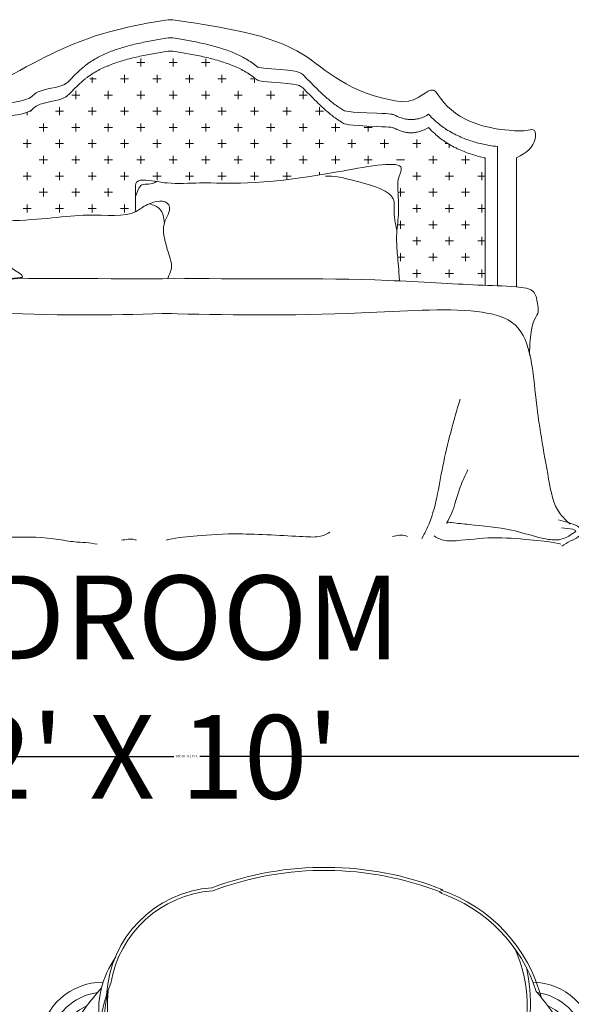
# Model space of a CAD drawing. Units: inches. Extents: x 1771 to 3025, y 319 to 889.
# Tile 22 of 35: x 2456 to 2502, y 703 to 786. Entities that reach past the tile are written whole.
import ezdxf

# ---------------------------------------------------------------- set-up
doc = ezdxf.new("R2010")
doc.units = ezdxf.units.IN
doc.header["$MEASUREMENT"] = 0
doc.set_wipeout_variables(frame=1)
for name, color, linetype, lineweight in [('A-ANNO-DIMS', 2, 'Continuous', 18), ('A-AREA-IDEN', 241, 'Continuous', 25), ('A-FURN', 8, 'Continuous', 18)]:
    doc.layers.add(name, color=color, linetype=linetype, lineweight=lineweight)
doc.styles.get("Standard").update_dxf_attribs({"font": 'arial.ttf'})
doc.dimstyles.get("Standard").update_dxf_attribs({"dimtxt": 0.18, "dimasz": 0.18, "dimexe": 0.18, "dimexo": 0.0625, "dimgap": 0.09, "dimtad": 0, "dimtih": 1, "dimtoh": 1, "dimdec": 4, "dimzin": 0, "dimdsep": 46, "dimtxsty": 'Standard', "dimcen": 0.09, "dimadec": 0, "dimazin": 0, "dimtfac": 1, "dimtdec": 4, "dimtofl": 0, "dimtmove": 0, "dimatfit": 3, "dimfxl": 1, "dimtolj": 1, "dimtzin": 0, "dimarcsym": 0})

# ---------------------------------------------------------------- blocks, each defined once
blk = doc.blocks.new('A$C3F6F0378')
for p, q in [((1198.7, 944.7), (1198.7, 946.2)), ((1254.2, 952.6), (1270.1, 952.6)), ((1262.2, 944.7), (1262.2, 960.5)), ((1317.7, 952.6), (1333.6, 952.6)), ((1325.7, 944.7), (1325.7, 960.5)), ((1381.2, 952.6), (1397.1, 952.6)), ((1389.2, 944.7), (1389.2, 959.9)), ((1230.4, 912.9), (1230.4, 928.8)), ((1293.9, 912.9), (1293.9, 928.8)), ((1357.4, 912.9), (1357.4, 928.8)), ((1420.9, 912.9), (1420.9, 928.8)), ((1162.7, 920.9), (1174.9, 920.9)), ((1166.9, 912.9), (1166.9, 924)), ((1222.5, 920.9), (1238.4, 920.9)), ((1286, 920.9), (1301.9, 920.9)), ((1349.5, 920.9), (1365.4, 920.9)), ((1413, 920.9), (1428.9, 920.9)), ((1476.5, 920.9), (1485.8, 920.9)), ((1484.4, 912.9), (1484.4, 921.6)), ((1127.2, 889.1), (1143.1, 889.1)), ((1135.2, 881.2), (1135.2, 897)), ((1190.7, 889.1), (1206.6, 889.1)), ((1198.7, 881.2), (1198.7, 897)), ((1254.2, 889.1), (1270.1, 889.1)), ((1262.2, 881.2), (1262.2, 897)), ((1317.7, 889.1), (1333.6, 889.1)), ((1325.7, 881.2), (1325.7, 897)), ((1381.2, 889.1), (1397.1, 889.1)), ((1389.2, 881.2), (1389.2, 897)), ((1444.7, 889.1), (1460.6, 889.1)), ((1452.7, 881.2), (1452.7, 897)), ((1508.2, 889.1), (1524.1, 889.1)), ((1516.2, 881.2), (1516.2, 897)), ((1571.7, 889.1), (1587.6, 889.1)), ((1579.7, 881.2), (1579.7, 897)), ((1039.9, 849.4), (1039.9, 855.2)), ((1044.6, 857.4), (1047.9, 857.4)), ((1095.5, 857.4), (1111.4, 857.4)), ((1103.4, 849.4), (1103.4, 865.3)), ((1159, 857.4), (1174.9, 857.4)), ((1166.9, 849.4), (1166.9, 865.3)), ((1222.5, 857.4), (1238.4, 857.4)), ((1230.4, 849.4), (1230.4, 865.3)), ((1286, 857.4), (1301.9, 857.4)), ((1293.9, 849.4), (1293.9, 865.3)), ((1349.5, 857.4), (1365.4, 857.4)), ((1357.4, 849.4), (1357.4, 865.3)), ((1413, 857.4), (1428.9, 857.4)), ((1420.9, 849.4), (1420.9, 865.3)), ((1476.5, 857.4), (1492.4, 857.4)), ((1484.4, 849.4), (1484.4, 865.3)), ((1540, 857.4), (1555.9, 857.4)), ((1547.9, 849.4), (1547.9, 865.3)), ((1603.5, 857.4), (1619.4, 857.4)), ((1611.4, 849.4), (1611.4, 865.3)), ((1071.7, 817.7), (1071.7, 833.5)), ((1135.2, 817.7), (1135.2, 833.5)), ((1198.7, 817.7), (1198.7, 833.5)), ((1262.2, 817.7), (1262.2, 833.5)), ((1325.7, 817.7), (1325.7, 833.5)), ((1389.2, 817.7), (1389.2, 833.5)), ((1452.7, 817.7), (1452.7, 833.5)), ((1516.2, 817.7), (1516.2, 833.5)), ((1579.7, 817.7), (1579.7, 833.5)), ((1643.2, 817.7), (1643.2, 833.5)), ((1063.7, 825.6), (1079.6, 825.6)), ((1127.2, 825.6), (1143.1, 825.6)), ((1190.7, 825.6), (1206.6, 825.6)), ((1254.2, 825.6), (1270.1, 825.6)), ((1317.7, 825.6), (1333.6, 825.6)), ((1381.2, 825.6), (1397.1, 825.6)), ((1444.7, 825.6), (1460.6, 825.6)), ((1508.2, 825.6), (1524.1, 825.6)), ((1571.7, 825.6), (1587.6, 825.6)), ((1635.2, 825.6), (1651.1, 825.6)), ((1698.7, 825.6), (1714.6, 825.6)), ((1706.7, 817.7), (1706.7, 828.2)), ((1770.2, 818.9), (1770.2, 818.9)), ((1032, 793.9), (1047.9, 793.9)), ((1039.9, 785.9), (1039.9, 801.8)), ((1095.5, 793.9), (1111.4, 793.9)), ((1103.4, 785.9), (1103.4, 801.8)), ((1159, 793.9), (1174.9, 793.9)), ((1166.9, 785.9), (1166.9, 801.8)), ((1222.5, 793.9), (1238.4, 793.9)), ((1230.4, 785.9), (1230.4, 801.8)), ((1286, 793.9), (1301.9, 793.9)), ((1293.9, 785.9), (1293.9, 801.8)), ((1349.5, 793.9), (1365.4, 793.9)), ((1357.4, 785.9), (1357.4, 801.8)), ((1413, 793.9), (1428.9, 793.9)), ((1420.9, 785.9), (1420.9, 801.8)), ((1476.5, 793.9), (1492.4, 793.9)), ((1484.4, 785.9), (1484.4, 801.8)), ((1540, 793.9), (1555.9, 793.9)), ((1547.9, 785.9), (1547.9, 801.8)), ((1603.5, 793.9), (1619.4, 793.9)), ((1611.4, 785.9), (1611.4, 801.8)), ((1667, 793.9), (1682.9, 793.9)), ((1674.9, 785.9), (1674.9, 801.8)), ((1730.5, 793.9), (1746.4, 793.9)), ((1738.4, 785.9), (1738.4, 801.8)), ((1794, 793.9), (1809.9, 793.9)), ((1801.9, 785.9), (1801.9, 801.8)), ((1857.5, 793.9), (1863, 793.9)), ((1865.4, 785.9), (1865.4, 792.4)), ((1063.7, 762.1), (1079.6, 762.1)), ((1071.7, 754.2), (1071.7, 770)), ((1127.2, 762.1), (1143.1, 762.1)), ((1135.2, 754.2), (1135.2, 770)), ((1190.7, 762.1), (1206.6, 762.1)), ((1198.7, 754.2), (1198.7, 770)), ((1254.2, 762.1), (1270.1, 762.1)), ((1262.2, 754.2), (1262.2, 770)), ((1317.7, 762.1), (1333.6, 762.1)), ((1325.7, 754.2), (1325.7, 770)), ((1381.2, 762.1), (1397.1, 762.1)), ((1389.2, 754.2), (1389.2, 770)), ((1444.7, 762.1), (1460.6, 762.1)), ((1452.7, 754.2), (1452.7, 770)), ((1508.2, 762.1), (1524.1, 762.1)), ((1516.2, 754.2), (1516.2, 770)), ((1571.7, 762.1), (1587.6, 762.1)), ((1579.7, 754.2), (1579.7, 770)), ((1635.2, 762.1), (1651.1, 762.1)), ((1643.2, 754.2), (1643.2, 770)), ((1698.7, 762.1), (1714.6, 762.1)), ((1706.7, 754.2), (1706.7, 770)), ((1762.2, 762.1), (1778.1, 762.1)), ((1825.7, 762.1), (1841.6, 762.1)), ((1833.7, 754.2), (1833.7, 770)), ((1889.2, 762.1), (1905.1, 762.1)), ((1897.2, 754.2), (1897.2, 770)), ((1039.9, 722.4), (1039.9, 738.3)), ((1103.4, 722.4), (1103.4, 738.3)), ((1166.9, 722.4), (1166.9, 738.3)), ((1230.4, 722.4), (1230.4, 738.3)), ((1293.9, 722.4), (1293.9, 738.3)), ((1357.4, 722.4), (1357.4, 738.3)), ((1420.9, 722.4), (1420.9, 738.3)), ((1484.4, 722.4), (1484.4, 738.3)), ((1547.9, 723.4), (1547.9, 738.3)), ((1611.4, 732.6), (1611.4, 738.3)), ((1801.9, 722.4), (1801.9, 738.3)), ((1865.4, 722.4), (1865.4, 738.3)), ((1928.9, 722.4), (1928.9, 738.3)), ((1032, 730.4), (1047.9, 730.4)), ((1095.5, 730.4), (1111.4, 730.4)), ((1159, 730.4), (1174.9, 730.4)), ((1222.5, 730.4), (1238.4, 730.4)), ((1286, 730.4), (1301.9, 730.4)), ((1349.5, 730.4), (1365.4, 730.4)), ((1413, 730.4), (1428.9, 730.4)), ((1476.5, 730.4), (1492.4, 730.4)), ((1540, 730.4), (1555.9, 730.4)), ((1794, 730.4), (1809.9, 730.4)), ((1857.5, 730.4), (1873.4, 730.4)), ((1921, 730.4), (1935.3, 730.4)), ((1063.7, 698.6), (1079.6, 698.6)), ((1071.7, 690.7), (1071.7, 706.5)), ((1127.2, 698.6), (1143.1, 698.6)), ((1135.2, 690.7), (1135.2, 706.5)), ((1190.7, 698.6), (1206.6, 698.6)), ((1198.7, 690.7), (1198.7, 706.5)), ((1765.2, 698.6), (1778.1, 698.6)), ((1770.2, 690.7), (1770.2, 706.5)), ((1825.7, 698.6), (1841.6, 698.6)), ((1833.7, 690.7), (1833.7, 706.5)), ((1889.2, 698.6), (1905.1, 698.6)), ((1897.2, 690.7), (1897.2, 706.5)), ((1039.9, 658.9), (1039.9, 674.8)), ((1103.4, 658.9), (1103.4, 674.8)), ((1166.9, 658.9), (1166.9, 674.8)), ((1230.4, 658.9), (1230.4, 674.8)), ((1801.9, 658.9), (1801.9, 674.8)), ((1865.4, 658.9), (1865.4, 674.8)), ((1928.9, 658.9), (1928.9, 674.8)), ((1032, 666.9), (1047.9, 666.9)), ((1095.5, 666.9), (1111.4, 666.9)), ((1159, 666.9), (1174.9, 666.9)), ((1222.5, 666.9), (1238.4, 666.9)), ((1794, 666.9), (1809.9, 666.9)), ((1857.5, 666.9), (1873.4, 666.9)), ((1921, 666.9), (1935.3, 666.9)), ((1770.2, 627.2), (1770.2, 643)), ((1833.7, 627.2), (1833.7, 643)), ((1897.2, 627.2), (1897.2, 643)), ((1764.2, 635.1), (1778.1, 635.1)), ((1825.7, 635.1), (1841.6, 635.1)), ((1889.2, 635.1), (1905.1, 635.1)), ((1794, 603.4), (1809.9, 603.4)), ((1801.9, 595.4), (1801.9, 611.3)), ((1857.5, 603.4), (1873.4, 603.4)), ((1865.4, 595.4), (1865.4, 611.3)), ((1921, 603.4), (1935.3, 603.4)), ((1928.9, 595.4), (1928.9, 611.3)), ((1770.2, 563.7), (1770.2, 579.5)), ((1833.7, 563.7), (1833.7, 579.5)), ((1897.2, 563.7), (1897.2, 579.5)), ((1764.5, 571.6), (1778.1, 571.6)), ((1825.7, 571.6), (1841.6, 571.6)), ((1889.2, 571.6), (1905.1, 571.6)), ((1794, 539.9), (1809.9, 539.9)), ((1801.9, 531.9), (1801.9, 547.8)), ((1857.5, 539.9), (1873.4, 539.9)), ((1865.4, 531.9), (1865.4, 547.8)), ((1921, 539.9), (1935.3, 539.9)), ((1928.9, 531.9), (1928.9, 547.8))]:
    blk.add_line(p, q)
at = {"ltscale": 20}
for p, q in [((1959.8, 788.3), (1959.8, 515.7)), ((1935.3, 766), (1935.3, 516.7)), ((1996.6, 766.2), (1996.6, 513.5))]:
    blk.add_line(p, q, dxfattribs=at)
for centre in [(1320.3, 981.3), (1320.4, 945.7), (1320.4, 919.9)]:
    blk.add_arc(centre, 55.2, 80.5605, 99.4395, dxfattribs=at)
for points, knots in [([(695.7, 766.2), (675.2, 775.8), (657.2, 791.6), (658.6, 824.3), (675.7, 817.9), (731.9, 819.9), (817.7, 836.7), (863.4, 913.8), (889.3, 869.9), (957.4, 896.6), (1128.9, 1003.6), (1245.7, 1025), (1311.4, 1035.8)], [12.417853, 12.417853, 12.417853, 12.417853, 68.394536, 90.665986, 114.156853, 157.554067, 281.869614, 298.858744, 338.737111, 347.060176, 470.423438, 625.498764, 625.498764, 625.498764, 625.498764]), ([(1996.6, 766.2), (2017.1, 775.8), (2035.1, 791.6), (2033.8, 824.3), (2016.6, 817.9), (1960.4, 819.9), (1874.7, 836.7), (1829, 913.8), (1803, 869.9), (1652.5, 896.6), (1584, 1003.6), (1395.1, 1025), (1329.4, 1035.8)], [12.417853, 12.417853, 12.417853, 12.417853, 68.394536, 90.665986, 114.156853, 157.554067, 281.869614, 298.858744, 338.737111, 347.060176, 470.423438, 625.498764, 625.498764, 625.498764, 625.498764]), ([(867.4, 851.3), (868.1, 850.9), (868.9, 850.4), (871.2, 849.1), (872.9, 848.2), (876.8, 846.3), (879, 845.4), (884, 843.6), (886.7, 842.8), (892, 841.7), (894.6, 841.4), (898.4, 841.1), (899.4, 841), (901.2, 841), (901.9, 841), (903.1, 841), (903.7, 841.1), (904.8, 841.1), (905.4, 841.2), (907, 841.3), (908.1, 841.4), (911.6, 841.9), (913.8, 842.3), (917.8, 843.3), (919.6, 843.9), (922.7, 844.9), (924.1, 845.5), (926.6, 846.4), (927.6, 846.9), (928.8, 847.4), (929.1, 847.5), (929.7, 847.8), (929.9, 847.9), (930.7, 848.2), (931.3, 848.5), (932.9, 849.2), (933.9, 849.7), (937.1, 851.3), (939.2, 852.3), (945.3, 855.5), (949.2, 857.8), (959.8, 864.4), (966.2, 869), (1040, 878.3), (1045.6, 883.1), (1056.3, 892.7), (1061.3, 897.5), (1112.2, 907), (1116.8, 911.6), (1125.6, 920.6), (1129.9, 924.9), (1138.3, 933), (1142.3, 936.8), (1148.2, 942), (1150, 943.5), (1153.3, 946.3), (1154.7, 947.4), (1157, 949.2), (1157.9, 949.9), (1159.7, 951.2), (1160.6, 951.8), (1163.4, 953.8), (1165.3, 955), (1171, 958.7), (1174.9, 961), (1186, 967), (1193.5, 970.4), (1209.3, 976.7), (1217.6, 979.5), (1235, 984.7), (1244, 987), (1262.7, 991.3), (1272.4, 993.3), (1291.8, 996.9), (1301.5, 998.6), (1311.3, 1000.2)], [328.6705, 328.6705, 328.6705, 328.6705, 329.609368, 329.609368, 331.487103, 331.487103, 333.620342, 333.620342, 335.753581, 335.753581, 337.507866, 337.507866, 338.182373, 338.182373, 338.607397, 338.607397, 338.959312, 338.959312, 339.311227, 339.311227, 340.015058, 340.015058, 341.722742, 341.722742, 343.430427, 343.430427, 345.138111, 345.138111, 346.845796, 346.845796, 347.37881, 347.37881, 347.911824, 347.911824, 348.977853, 348.977853, 351.109909, 351.109909, 355.374023, 355.374023, 363.902249, 363.902249, 379.258481, 379.258481, 394.614712, 394.614712, 409.970944, 409.970944, 425.327175, 425.327175, 440.683406, 440.683406, 456.039638, 456.039638, 463.285514, 463.285514, 469.01116, 469.01116, 472.593, 472.593, 476.17484, 476.17484, 483.338521, 483.338521, 497.665882, 497.665882, 522.309302, 522.309302, 546.952723, 546.952723, 571.596143, 571.596143, 596.239564, 596.239564, 619.876409, 619.876409, 619.876409, 619.876409]), ([(1824.9, 851.3), (1824.2, 850.9), (1823.5, 850.4), (1821.1, 849.1), (1819.5, 848.2), (1815.6, 846.3), (1813.3, 845.4), (1808.4, 843.6), (1805.7, 842.8), (1800.3, 841.7), (1797.7, 841.4), (1794, 841.1), (1792.9, 841), (1791.2, 841), (1790.5, 841), (1789.2, 841), (1788.6, 841.1), (1787.5, 841.1), (1787, 841.2), (1785.3, 841.3), (1784.3, 841.4), (1780.8, 841.9), (1778.6, 842.3), (1774.6, 843.3), (1772.8, 843.9), (1769.6, 844.9), (1768.2, 845.5), (1765.8, 846.4), (1764.7, 846.9), (1763.5, 847.4), (1763.2, 847.5), (1762.7, 847.8), (1762.4, 847.9), (1761.6, 848.2), (1761.1, 848.5), (1759.5, 849.2), (1758.4, 849.7), (1755.2, 851.3), (1753.2, 852.3), (1664.6, 855.5), (1660.7, 857.8), (1650.1, 864.4), (1643.7, 869), (1631.7, 878.3), (1626.1, 883.1), (1615.5, 892.7), (1610.4, 897.5), (1600.8, 907), (1596.2, 911.6), (1587.3, 920.6), (1583, 924.9), (1574.7, 933), (1570.6, 936.8), (1492.6, 942), (1490.8, 943.5), (1487.5, 946.3), (1486.1, 947.4), (1483.8, 949.2), (1482.9, 949.9), (1481.1, 951.2), (1480.2, 951.8), (1477.4, 953.8), (1475.5, 955), (1469.8, 958.7), (1465.9, 961), (1454.8, 967), (1447.3, 970.4), (1431.5, 976.7), (1423.2, 979.5), (1405.8, 984.7), (1396.8, 987), (1378.1, 991.3), (1368.4, 993.3), (1349, 996.9), (1339.3, 998.6), (1329.5, 1000.2)], [328.6705, 328.6705, 328.6705, 328.6705, 329.609368, 329.609368, 331.487103, 331.487103, 333.620342, 333.620342, 335.753581, 335.753581, 337.507866, 337.507866, 338.182373, 338.182373, 338.607397, 338.607397, 338.959312, 338.959312, 339.311227, 339.311227, 340.015058, 340.015058, 341.722742, 341.722742, 343.430427, 343.430427, 345.138111, 345.138111, 346.845796, 346.845796, 347.37881, 347.37881, 347.911824, 347.911824, 348.977853, 348.977853, 351.109909, 351.109909, 355.374023, 355.374023, 363.902249, 363.902249, 379.258481, 379.258481, 394.614712, 394.614712, 409.970943, 409.970943, 425.327175, 425.327175, 440.683406, 440.683406, 456.039637, 456.039637, 463.285514, 463.285514, 469.011154, 469.011154, 472.592992, 472.592992, 476.17483, 476.17483, 483.338506, 483.338506, 497.665857, 497.665857, 522.309275, 522.309275, 546.952693, 546.952693, 571.59611, 571.59611, 596.239528, 596.239528, 619.876409, 619.876409, 619.876409, 619.876409]), ([(867.4, 825.4), (868.1, 825), (868.9, 824.6), (871.2, 823.2), (872.9, 822.3), (876.8, 820.5), (879, 819.5), (884, 817.8), (886.7, 817), (892, 815.9), (894.6, 815.5), (898.4, 815.2), (899.4, 815.2), (901.2, 815.2), (901.9, 815.2), (903.1, 815.2), (903.7, 815.2), (904.8, 815.3), (905.4, 815.3), (907, 815.4), (908.1, 815.5), (911.6, 816), (913.8, 816.5), (917.8, 817.5), (919.6, 818), (922.7, 819.1), (924.1, 819.6), (926.6, 820.6), (927.6, 821), (928.8, 821.5), (929.1, 821.7), (929.7, 821.9), (929.9, 822), (930.7, 822.4), (931.3, 822.6), (932.9, 823.4), (933.9, 823.9), (937.1, 825.4), (939.2, 826.4), (945.3, 829.7), (949.2, 832), (959.8, 838.6), (966.2, 843.1), (1040, 852.4), (1045.6, 857.2), (1056.3, 866.8), (1061.3, 871.6), (1112.2, 881.1), (1116.8, 885.7), (1125.6, 894.7), (1129.9, 899), (1138.3, 907.1), (1142.3, 910.9), (1148.2, 916.1), (1150, 917.7), (1153.3, 920.4), (1154.7, 921.5), (1157, 923.3), (1157.9, 924), (1159.7, 925.3), (1160.6, 926), (1163.4, 927.9), (1165.3, 929.2), (1171, 932.8), (1174.9, 935.2), (1186, 941.1), (1193.5, 944.6), (1209.3, 950.8), (1217.6, 953.7), (1235, 958.8), (1244, 961.2), (1262.7, 965.5), (1272.4, 967.4), (1291.8, 971), (1301.5, 972.7), (1311.3, 974.3)], [328.6705, 328.6705, 328.6705, 328.6705, 329.609368, 329.609368, 331.487103, 331.487103, 333.620342, 333.620342, 335.753581, 335.753581, 337.507866, 337.507866, 338.182373, 338.182373, 338.607397, 338.607397, 338.959312, 338.959312, 339.311227, 339.311227, 340.015058, 340.015058, 341.722742, 341.722742, 343.430427, 343.430427, 345.138111, 345.138111, 346.845796, 346.845796, 347.37881, 347.37881, 347.911824, 347.911824, 348.977853, 348.977853, 351.109909, 351.109909, 355.374023, 355.374023, 363.902249, 363.902249, 379.258481, 379.258481, 394.614712, 394.614712, 409.970944, 409.970944, 425.327175, 425.327175, 440.683406, 440.683406, 456.039638, 456.039638, 463.285514, 463.285514, 469.01116, 469.01116, 472.593, 472.593, 476.17484, 476.17484, 483.338521, 483.338521, 497.665882, 497.665882, 522.309302, 522.309302, 546.952723, 546.952723, 571.596143, 571.596143, 596.239564, 596.239564, 619.876409, 619.876409, 619.876409, 619.876409]), ([(1824.9, 825.4), (1824.2, 825), (1823.5, 824.6), (1821.1, 823.2), (1819.5, 822.3), (1815.6, 820.5), (1813.3, 819.5), (1808.4, 817.8), (1805.7, 817), (1800.3, 815.9), (1797.7, 815.5), (1794, 815.2), (1792.9, 815.2), (1791.2, 815.2), (1790.5, 815.2), (1789.2, 815.2), (1788.6, 815.2), (1787.5, 815.3), (1787, 815.3), (1785.3, 815.4), (1784.3, 815.5), (1780.8, 816), (1778.6, 816.5), (1774.6, 817.5), (1772.8, 818), (1769.6, 819.1), (1768.2, 819.6), (1765.8, 820.6), (1764.7, 821), (1763.5, 821.5), (1763.2, 821.7), (1762.7, 821.9), (1762.4, 822), (1761.6, 822.4), (1761.1, 822.6), (1759.5, 823.4), (1758.4, 823.9), (1755.2, 825.4), (1753.2, 826.4), (1664.6, 829.7), (1660.7, 832), (1650.1, 838.6), (1643.7, 843.1), (1631.7, 852.4), (1626.1, 857.2), (1615.5, 866.8), (1610.4, 871.6), (1600.8, 881.1), (1596.2, 885.7), (1587.3, 894.7), (1583, 899), (1574.7, 907.1), (1570.6, 910.9), (1492.6, 916.1), (1490.8, 917.7), (1487.5, 920.4), (1486.1, 921.5), (1483.8, 923.3), (1482.9, 924), (1481.1, 925.3), (1480.2, 926), (1477.4, 927.9), (1475.5, 929.2), (1469.8, 932.8), (1465.9, 935.2), (1454.8, 941.1), (1447.3, 944.6), (1431.5, 950.8), (1423.2, 953.7), (1405.8, 958.8), (1396.8, 961.2), (1378.1, 965.5), (1368.4, 967.4), (1349, 971), (1339.3, 972.7), (1329.5, 974.3)], [328.6705, 328.6705, 328.6705, 328.6705, 329.609368, 329.609368, 331.487103, 331.487103, 333.620342, 333.620342, 335.753581, 335.753581, 337.507866, 337.507866, 338.182373, 338.182373, 338.607397, 338.607397, 338.959312, 338.959312, 339.311227, 339.311227, 340.015058, 340.015058, 341.722742, 341.722742, 343.430427, 343.430427, 345.138111, 345.138111, 346.845796, 346.845796, 347.37881, 347.37881, 347.911824, 347.911824, 348.977853, 348.977853, 351.109909, 351.109909, 355.374023, 355.374023, 363.902249, 363.902249, 379.258481, 379.258481, 394.614712, 394.614712, 409.970943, 409.970943, 425.327175, 425.327175, 440.683406, 440.683406, 456.039637, 456.039637, 463.285514, 463.285514, 469.011154, 469.011154, 472.592992, 472.592992, 476.17483, 476.17483, 483.338506, 483.338506, 497.665857, 497.665857, 522.309275, 522.309275, 546.952693, 546.952693, 571.59611, 571.59611, 596.239528, 596.239528, 619.876409, 619.876409, 619.876409, 619.876409]), ([(1959.8, 788.3), (1947.6, 789.5), (1939.9, 790.9), (1923.7, 794.5), (1915.4, 796.7), (1898.5, 802.3), (1889.9, 805.7), (1873, 813.7), (1864.6, 818.4), (1849.7, 828.5), (1843.2, 833.6), (1832.8, 843.1), (1828.8, 847.1), (1824.9, 851.3)], [179.400376, 179.400376, 179.400376, 179.400376, 196.086144, 196.086144, 213.445516, 213.445516, 230.804888, 230.804888, 248.16426, 248.16426, 262.451931, 262.451931, 271.832526, 271.832526, 271.832526, 271.832526]), ([(1935.3, 766), (1934.2, 766.3), (1933.1, 766.5), (1923.7, 768.6), (1915.4, 770.9), (1898.5, 776.5), (1889.9, 779.8), (1873, 787.9), (1864.6, 792.6), (1849.7, 802.7), (1843.2, 807.8), (1832.8, 817.2), (1828.8, 821.2), (1824.9, 825.4)], [193.740688, 193.740688, 193.740688, 193.740688, 196.086144, 196.086144, 213.445516, 213.445516, 230.804888, 230.804888, 248.16426, 248.16426, 262.451931, 262.451931, 271.832526, 271.832526, 271.832526, 271.832526])]:
    blk.add_open_spline(points, degree=3, knots=knots, dxfattribs=at)
at = {"ltscale": 5}
for points, knots in [([(1251.5, 660.5), (1251.8, 673.8), (1252.2, 692.2), (1250.9, 722.8), (1282.7, 722.3), (1319.1, 713.9), (1424.2, 721.3), (1489.1, 705.6), (1786.5, 765.5), (1764.9, 728.8), (1764.7, 698.2), (1767.9, 658.9), (1761, 614.3), (1764.1, 574.4), (1766.6, 548.7), (1767.9, 525.2)], [3.603347, 3.603347, 3.603347, 3.603347, 60.838375, 82.182907, 107.012175, 163.177093, 249.239778, 501.114283, 577.787612, 607.274607, 630.949286, 706.159707, 762.92633, 812.910096, 867.096105, 867.096105, 867.096105, 867.096105]), ([(1293.1, 719.7), (1288.2, 716.8), (1279.1, 713), (1263.5, 715.9), (1256.5, 703.2), (1253.3, 695), (1251.9, 690.7)], [16.588235, 16.588235, 16.588235, 16.588235, 39.368234, 56.465167, 72.647278, 91.317886, 91.317886, 91.317886, 91.317886]), ([(1623.4, 730.2), (1631.2, 730.2), (1644.4, 730.3), (1665.2, 725.1), (1763.6, 700.2), (1754.4, 664.8), (1760.1, 637.6), (1763, 624), (1763.1, 623.6)], [0, 0, 0, 0, 31.268494, 53.71641, 83.24833, 138.583941, 192.96698, 194.695488, 194.695488, 194.695488, 194.695488]), ([(964.3, 525.7), (965, 536.9), (1030.6, 547.7), (956.6, 565.4), (948, 599.2), (929.2, 612.7), (925.7, 647.1), (951.8, 642.5), (1054.9, 642.1), (1162.4, 661.2), (1239, 646.9), (1276.3, 678.9), (1316.3, 686.5), (1319.5, 660.6), (1309.9, 647.1), (1305, 623.9), (1309.2, 608.7), (1312.5, 586.6), (1326.7, 553.1), (1318.1, 538.8), (1314.8, 529.7)], [33.020195, 33.020195, 33.020195, 33.020195, 57.294753, 90.473933, 194.149416, 257.058105, 304.592565, 338.383824, 389.043604, 577.649845, 759.359611, 813.032269, 898.973184, 920.659088, 956.429806, 1000.911745, 1042.797508, 1121.842246, 1191.460876, 1213.109701, 1213.109701, 1213.109701, 1213.109701]), ([(1278.5, 676.1), (1286.8, 673.9), (1304.1, 667.4), (1307.6, 649.1), (1308.3, 637.8)], [13.535772, 13.535772, 13.535772, 13.535772, 45.871957, 87.312392, 87.312392, 87.312392, 87.312392]), ([(961.3, 642.9), (955.5, 638.3), (944, 626.2), (1030.7, 599.4), (953, 567.4), (1038.4, 539.7), (1029.3, 530.5), (966, 529.3)], [5.952535, 5.952535, 5.952535, 5.952535, 29.258845, 70.114919, 115.518645, 162.322231, 169.813565, 169.813565, 169.813565, 169.813565]), ([(643.4, 331.9), (665.9, 445.8), (654.5, 454.3), (658, 480.9), (661.2, 509.9), (714.1, 515.4), (786.5, 516.7), (1040.5, 536.6), (1224.6, 526.5), (1352.9, 530.4)], [0, 0, 0, 0, 32.681627, 48.455722, 75.25348, 112.004017, 183.381957, 310.642358, 688.088714, 688.088714, 688.088714, 688.088714]), ([(2022.3, 380), (2023.2, 448.3), (2041.3, 454.3), (2037.8, 480.9), (2034.7, 509.9), (1981.7, 515.4), (1909.3, 516.7), (1667.8, 533.2), (1476.1, 527.9), (1347.4, 530.2)], [0, 0, 0, 0, 32.681627, 48.455722, 75.25348, 112.004017, 183.381957, 310.642358, 588.939547, 588.939547, 588.939547, 588.939547]), ([(594.1, 49), (601.1, 55.3), (626, 78.1), (628.7, 172), (631.8, 287.1), (663.1, 436.6), (808.3, 475), (1037.5, 455.3), (1227.9, 458.5), (1322.1, 461.7)], [0, 0, 0, 0, 28.320233, 100.953775, 269.820348, 420.691469, 489.161544, 656.134073, 940.569207, 940.569207, 940.569207, 940.569207]), ([(2101.8, 49), (2094.8, 55.3), (2069.8, 78.1), (2053.9, 172), (2031.7, 287.1), (2023.3, 445.1), (1887.5, 475), (1637.7, 455.3), (1416.4, 458.5), (1314.5, 461.4)], [0, 0, 0, 0, 28.320233, 100.953775, 269.820348, 420.691469, 489.161544, 656.134073, 940.569207, 940.569207, 940.569207, 940.569207]), ([(1886.4, 293.6), (1874, 250.4), (1850.2, 167.7), (1838.6, 71.7), (1815.4, 27.8), (1811.5, 20.4)], [0, 0, 0, 0, 135.247847, 258.692787, 283.800228, 283.800228, 283.800228, 283.800228]), ([(1901.7, 155.1), (1896.3, 144.1), (1881.1, 112.8), (1874.4, 74.6), (1861.4, 53), (1859.9, 50.7)], [0, 0, 0, 0, 37.234018, 105.386078, 113.844905, 113.844905, 113.844905, 113.844905]), ([(2080.3, 18.4), (2075.6, 18.3), (2062.2, 17.9), (2030.9, 24.9), (1978.8, 41.9), (1919.5, 46.5), (1879.3, 50.9), (1863, 53.1), (1860.4, 51), (1859.9, 50.7)], [0, 0, 0, 0, 14.447875, 40.468341, 96.220884, 181.018327, 216.046098, 224.609189, 226.185962, 226.185962, 226.185962, 226.185962]), ([(2084.9, 41.8), (2100.9, 40.1), (2120.5, 38.1), (2104.4, 29.7), (2095.5, 21.9), (2085.1, 19.8), (2078.6, 18.4)], [0, 0, 0, 0, 28.05485, 34.289435, 45.980108, 65.027556, 65.027556, 65.027556, 65.027556]), ([(2079, 57.4), (2084.9, 55.8), (2100.2, 51.8), (2131, 40.6), (2116.7, 21.1), (2101.3, 16.6), (2091, 9.7), (2085.5, 5.9)], [0, 0, 0, 0, 19.937155, 51.57724, 63.193909, 80.21631, 100.09061, 100.09061, 100.09061, 100.09061]), ([(815.7, 37.2), (795, 34.1), (767.8, 30.1), (693.6, 25.5), (716, 16.2), (729.8, 21.8), (754.8, 20), (787, 17), (826.3, 22.8), (869.3, 25.1), (905.1, 21.9), (935.5, 27.3), (1029.7, 21.6), (1063.4, 26), (1134.3, 13.3), (1155.4, 13.6), (1169.6, 10.9), (1177, 9.9)], [0, 0, 0, 0, 87.513803, 114.592793, 124.77702, 141.903576, 160.817021, 198.691115, 240.471478, 280.23486, 329.410006, 348.41762, 373.077233, 428.05708, 447.802257, 468.691939, 491.310217, 491.310217, 491.310217, 491.310217]), ([(1224.5, 17.5), (1233.4, 18.9), (1243.5, 21.4), (1252.6, 17.9), (1253.7, 17.5)], [516.212662, 516.212662, 516.212662, 516.212662, 542.681017, 546.007116, 546.007116, 546.007116, 546.007116]), ([(1311.8, 17.5), (1313.3, 17.9), (1334, 23.1), (1377.5, 26.3), (1445.4, 32.7), (1573.8, 24.6), (1614, 23), (1627.1, 30.7), (1632, 33.6)], [590.079786, 590.079786, 590.079786, 590.079786, 594.646549, 651.888327, 725.747367, 797.841373, 826.274406, 843.189267, 843.189267, 843.189267, 843.189267]), ([(1754.5, 25.1), (1763.4, 26.5), (1773.5, 29), (1782.6, 25.5), (1783.6, 25.1)], [516.212662, 516.212662, 516.212662, 516.212662, 542.681017, 546.007116, 546.007116, 546.007116, 546.007116]), ([(2083.5, 9.9), (2082, 10.3), (2061.3, 15.5), (2017.8, 18.7), (1949.9, 25.1), (1893.7, 17), (1853.5, 15.4), (1840.4, 23.1), (1835.5, 26)], [590.079786, 590.079786, 590.079786, 590.079786, 594.646549, 651.888327, 725.747367, 797.841373, 826.274406, 843.189267, 843.189267, 843.189267, 843.189267])]:
    blk.add_open_spline(points, degree=3, knots=knots, dxfattribs=at)
blk = doc.blocks.new('A$C425441F1')
for points in [[(1639.3, 0), (1667.3, 0), (1667.3, 55.3), (1748.6, 55.3), (1748.6, 807.4), (1761.1, 860.7), (1735.7, 880.7), (1703.4, 883.3), (1675.8, 879.6), (1656.2, 873.5), (1635.2, 863.3), (1619.6, 852.6), (1605.1, 839.5), (1596.7, 829.9), (1583.2, 810), (1573.2, 788.1), (1567.6, 767.7), (1566.5, 761.6), (1541.6, 750.9), (1510.7, 736.6), (1488.3, 725.3), (1464.5, 712.2), (1433.4, 693.6), (1409.1, 677.8), (1389.7, 664.2), (1388.2, 683.8), (1383.3, 700), (1376.2, 712), (1365.5, 723.2), (1352, 731.8), (1342.1, 735.4), (1331.7, 738.6), (1325, 742.7), (1317.7, 750.9), (1314.2, 758.8), (1312.9, 767.9), (1315.6, 780.8), (1321.1, 788.9), (1323.4, 793.7), (1323.6, 797.2), (1323.1, 800), (1320.5, 804.5), (1317.8, 806.7), (1317.8, 807.1), (1478.8, 807.1), (1345.8, 1080.7), (1177.3, 1080.7), (1044.3, 807.1), (1211.1, 807.1), (1211.1, 806.7), (1207.8, 803.9), (1205.8, 800.4), (1205.1, 796.3), (1207.6, 788.9), (1211.4, 783.4), (1213.5, 778.7), (1215.3, 769.8), (1215.1, 763.9), (1214.1, 759), (1208.8, 748.5), (1201.9, 741.7), (1195.3, 738), (1185.9, 735.4), (1176, 731.7), (1166.8, 726.4), (1159.9, 720.8), (1156.8, 717.7), (1149.3, 708.1), (1145.7, 701.6), (1143.6, 696.9), (1138.7, 669.7), (1138.7, 651.6), (1140.7, 631.8), (1142.6, 621.6), (1148.5, 600.5), (1162.8, 569), (1176.9, 547.8), (1188.6, 534.2), (1200, 523), (983, 523), (977.7, 522.3), (971.8, 519.6), (965.5, 512.8), (963.3, 506.8), (963, 503), (974.8, 503), (974.8, 3), (1013, 3), (1013, 103), (1053.6, 103), (1052.7, 96.1), (1051.6, 86.5), (1049.3, 63.6), (1048.6, 55.3), (1130.1, 55.3), (1130.1, 0), (1157.9, 0), (1174.1, 55.3), (1623.1, 55.6)], [(778.6, 0), (750.6, 0), (750.6, 50.4), (141.4, 50.4), (141.4, 0), (113.4, 0), (98.1, 50.4), (0, 50.4), (0, 590.4), (3.6, 609.1), (14.7, 633.7), (36.6, 658.7), (60.6, 673.3), (86.6, 680.5), (100.5, 681.5), (107.8, 698), (118.3, 717), (136.4, 751.3), (159.1, 779.5), (188.4, 803.6), (213.2, 817.4), (239.4, 827.1), (258.7, 831.4), (276, 833.4), (301.1, 842.1), (332.2, 850.9), (368.4, 858.6), (403.3, 863.5), (432.7, 865.8), (472.6, 866.2), (499.3, 864.8), (525, 862.1), (551.9, 857.9), (572.9, 853.6), (591.1, 849.1), (612.6, 842.8), (648, 830.4), (661.5, 823.7), (679.5, 815.2), (707.5, 798.2), (726.7, 783.3), (755.4, 754.4), (773.7, 729.8), (788.1, 704.9), (796.6, 686.1), (798.5, 681.2), (818, 677.9), (833.5, 672.3), (851.7, 661.6), (864.4, 650.3), (878.3, 632.1), (887.5, 611.7), (891.4, 595.2), (892, 590.4), (892, 50.4), (793.9, 50.4)]]:
    blk.add_wipeout(points)
for p, q in [((1044.3, 807.1), (1177.3, 1080.7)), ((1177.3, 1080.7), (1044.3, 807.1)), ((1177.3, 1080.7), (1345.8, 1080.7)), ((1345.8, 1080.7), (1177.3, 1080.7)), ((1345.8, 1080.7), (1478.8, 807.1)), ((1478.8, 807.1), (1345.8, 1080.7)), ((1188.8, 1068), (1069.3, 827.4)), ((1201.1, 1068), (1081.6, 827.4)), ((1211.2, 1068), (1091.7, 827.4)), ((1223.5, 1068), (1104, 827.4)), ((1230.5, 1068), (1110.9, 827.4)), ((1242.8, 1068), (1123.2, 827.4)), ((1171, 1067.8), (1351.9, 1067.8)), ((1299.6, 1068), (1419.2, 827.4)), ((1311.9, 1068), (1431.5, 827.4)), ((1322, 1068), (1441.5, 827.4)), ((1334.3, 1068), (1453.8, 827.4)), ((1733.6, 876.1), (1755.5, 858.7)), ((1735.7, 880.7), (1761.1, 860.7)), ((1744.1, 810.1), (1755.5, 858.7)), ((1748.6, 807.4), (1761.1, 860.7)), ((1053.8, 826.7), (1469.3, 826.7)), ((1478.8, 807.1), (1044.3, 807.1)), ((1044.3, 807.1), (1478.8, 807.1)), ((1205.6, 800), (1323.1, 800)), ((1211, 806.7), (1317.8, 806.7)), ((1743.6, 60.3), (1743.6, 805)), ((1748.6, 55.3), (1748.6, 807.4)), ((18.2, 603.6), (18.2, 536.8)), ((0, 590.4), (0, 50.4)), ((15, 591.1), (15, 521.6)), ((31, 569.9), (31, 588.4)), ((861, 569.9), (861, 588.4)), ((877, 591.1), (877, 521.6)), ((892, 590.4), (892, 50.4)), ((1238.2, 523), (983, 523)), ((1222, 503), (963, 503)), ((974.8, 3), (974.8, 503)), ((1206.8, 483), (974.8, 483)), ((1013, 3), (1013, 483)), ((10, 417.4), (32, 265.4)), ((882, 417.4), (860, 265.4)), ((1092.2, 423), (974.8, 423)), ((15, 385.1), (15, 50.4)), ((877, 385.1), (877, 50.4)), ((1055.6, 314.3), (1046.6, 240.3)), ((1060.1, 309.3), (1051.6, 239.7)), ((1111.1, 314.3), (1055.6, 314.3)), ((1109, 309.3), (1060.1, 309.3)), ((31, 50.4), (31, 272.3)), ((861, 50.4), (861, 272.3)), ((276.3, 240.8), (286.9, 216)), ((589.2, 240.9), (599.9, 216.1)), ((245.5, 223.1), (286.9, 216)), ((558.4, 223.2), (599.9, 216.1)), ((108.8, 209.4), (790.1, 209.4)), ((109.6, 209.4), (783, 209.4)), ((286.9, 216), (276.9, 175.2)), ((286.9, 216), (298.3, 173.5)), ((599.9, 216.1), (589.8, 175.3)), ((599.9, 216.1), (611.2, 173.6)), ((109.6, 199.4), (783, 199.4)), ((285.7, 179.9), (278.3, 201.7)), ((598.7, 180), (591.2, 201.8)), ((298.3, 173.5), (285.7, 179.9)), ((611.2, 173.6), (598.7, 180)), ((31.6, 128.4), (31.6, 131.4)), ((41.6, 128.4), (41.6, 131.4)), ((851, 131.4), (851, 128.4)), ((861, 131.4), (861, 128.4)), ((1056.5, 123), (1013, 123)), ((1053.6, 103), (1013, 103)), ((0, 50.4), (892, 50.4)), ((113.4, 0), (97.2, 53.4)), ((783, 60.4), (109.6, 60.4)), ((783, 50.4), (109.6, 50.4)), ((141.4, 50.4), (141.4, 0)), ((750.6, 50.4), (750.6, 0)), ((778.6, 0), (794.8, 53.4)), ((1048.6, 55.3), (1748.6, 55.3)), ((1054, 60.3), (1743.6, 60.3)), ((1129.9, 52.6), (1129.9, 0)), ((1157.9, 0), (1174.2, 55.6)), ((1639.3, 0), (1623.1, 55.6)), ((1667.3, 52.6), (1667.3, 0)), ((141.4, 0), (113.4, 0)), ((750.6, 0), (778.6, 0)), ((1129.9, 0), (1157.9, 0)), ((1667.3, 0), (1639.3, 0))]:
    blk.add_line(p, q)
for centre, radius, start, end in [((1708.4, 739.8), 143.6, 79.0486, 171.2543), ((1708.4, 739.8), 138.6, 79.5487, 170.0411), ((458.1, 348.7), 517.8, 68.4843, 110.5916), ((458.1, 348.7), 512.8, 68.4843, 110.5916), ((289.3, 651.4), 182.6, 93.9855, 176.965), ((289.3, 651.4), 177.6, 93.9855, 170.8791), ((563, 591.9), 246.9, 17.5917, 71.2419), ((563, 591.9), 251.9, 14.3659, 71.2419), ((1873.1, -6.5), 826.8, 98.9741, 175.711), ((1873.1, -6.5), 821.8, 99.0642, 175.3352), ((1217.2, 796.3), 12.1, 120.8914, 217.6223), ((1311.5, 796.3), 12.1, 322.3777, 59.1086), ((1183, 767.9), 32.3, 282.2329, 40.4775), ((1345.2, 767.9), 32.3, 135.1029, 257.7671), ((560.7, 643.7), 223.1, 296.1387, 23.9967), ((1203.5, 673.6), 64.2, 102.2329, 173.5671), ((1324.7, 673.6), 64.2, 6.4329, 77.7671), ((242.1, 635.9), 148, 144.2704, 189.5276), ((512.5, 645.7), 276.4, 357.4515, 12.4082), ((100.5, 580.5), 100.9, 89.5113, 174.4069), ((508.9, 316.7), 542.9, 139.0716, 146.5815), ((333.5, 586), 238.7, 156.9166, 219.7497), ((331.3, 643.7), 223.1, 173.6107, 243.8613), ((791.5, 580.5), 100.9, 5.5931, 89.1441), ((383.1, 316.7), 542.9, 33.4185, 40.1113), ((1322.1, 660.2), 183.7, 173.5671, 228.321), ((1206.1, 660.2), 183.7, 1.2452, 6.4329), ((104.5, 574.5), 91, 97.7735, 169.4907), ((316.8, 619.2), 213.4, 167.2983, 240.5749), ((787.5, 574.5), 91, 10.5093, 82.2265), ((104.5, 574.5), 74.8, 113.0142, 169.2704), ((787.5, 574.5), 74.8, 10.7296, 66.9858), ((579.4, 614.6), 207.2, 299.0365, 4.5654), ((578.1, 577), 217.9, 318.7723, 15.0106), ((301.8, 453.4), 294.8, 146.5815, 180), ((590.2, 453.4), 294.8, 0, 33.4185), ((983, 503), 20, 90, 180), ((48.3, 453.8), 40.5, 46.9039, 174.9451), ((843.7, 453.8), 40.5, 5.0549, 133.0961), ((56.7, 434.2), 49.4, 95.5103, 189.1585), ((49, 344.1), 139.3, 24.2628, 91.6479), ((843, 344.1), 139.3, 88.3521, 155.7372), ((835.3, 434.2), 49.4, 350.8415, 84.4897), ((1177.9, 391.7), 91.3, 73.3794, 227.0029), ((1177.9, 391.7), 86.3, 74.5383, 225.8439), ((468.1, -775.2), 1235.6, 77.9993, 104.2473), ((423.9, -775.2), 1235.6, 75.7527, 102.0007), ((301.8, 453.4), 294.8, 180, 193.379), ((590.2, 453.4), 294.8, 346.621, 0), ((52.4, 315.2), 153.2, 329.9033, 50.4478), ((839.6, 315.2), 153.2, 129.5522, 210.0967), ((92.5, 308.8), 126.8, 335.5815, 48.2351), ((799.5, 308.8), 126.8, 131.7649, 204.4185), ((114.7, 252.6), 85.8, 14.0074, 167.3648), ((135.5, 294.2), 81.5, 277.3995, 32.8179), ((756.5, 294.2), 81.5, 147.1821, 262.6005), ((777.3, 252.6), 85.8, 12.6352, 165.9926), ((106.2, 240.2), 87.4, 106.4444, 125.4727), ((114.5, 212.1), 116.8, 90, 106.4444), ((114.5, 212.1), 116.8, 73.5556, 90), ((122.8, 240.2), 87.4, 54.5273, 73.5556), ((769.2, 240.2), 87.4, 106.4444, 125.4727), ((777.5, 212.1), 116.8, 90, 106.4444), ((777.5, 212.1), 116.8, 73.5556, 90), ((785.8, 240.2), 87.4, 54.5273, 73.5556), ((93.5, 258.1), 65.5, 125.4727, 149.8309), ((135.5, 258.1), 65.5, 30.1691, 54.5273), ((756.5, 258.1), 65.5, 125.4727, 149.8309), ((798.5, 258.1), 65.5, 30.1691, 54.5273), ((74.1, 269.4), 43.1, 149.8309, 180), ((154.9, 269.4), 43.1, 0, 30.1691), ((737.1, 269.4), 43.1, 149.8309, 180), ((817.9, 269.4), 43.1, 0, 30.1691), ((74.1, 269.4), 43.1, 180, 210.1691), ((154.9, 269.4), 43.1, 329.8309, 0), ((737.1, 269.4), 43.1, 180, 210.1691), ((817.9, 269.4), 43.1, 329.8309, 0), ((93.5, 280.6), 65.5, 210.1691, 234.5273), ((135.5, 280.6), 65.5, 305.4727, 329.8309), ((756.5, 280.6), 65.5, 210.1691, 234.5273), ((798.5, 280.6), 65.5, 305.4727, 329.8309), ((1071.6, 237.3), 25.1, 173.0657, 279.7438), ((1071.6, 237.3), 20.1, 173.0657, 286.6808), ((106.2, 298.5), 87.4, 234.5273, 253.5556), ((122.8, 298.5), 87.4, 286.4444, 305.4727), ((302.4, 220.7), 12.2, 53.3958, 216.551), ((615.4, 220.8), 12.2, 53.3958, 216.551), ((769.2, 298.5), 87.4, 234.5273, 253.5556), ((785.8, 298.5), 87.4, 286.4444, 305.4727), ((109.6, 131.4), 78, 90, 180), ((114.5, 326.6), 116.8, 253.5556, 270), ((114.5, 326.6), 116.8, 270, 286.4444), ((294.4, 177.6), 35.9, 92.8846, 181.9), ((607.4, 177.7), 35.9, 92.8846, 181.9), ((777.5, 326.6), 116.8, 253.5556, 270), ((777.5, 326.6), 116.8, 270, 286.4444), ((783, 131.4), 78, 0, 90), ((109.6, 131.4), 68, 90, 180), ((783, 131.4), 68, 0, 90), ((271.5, 234.5), 59.6, 257.4358, 275.1883), ((584.4, 234.6), 59.6, 257.4358, 275.1883), ((109.6, 128.4), 78, 180, 270), ((109.6, 128.4), 68, 180, 270), ((783, 128.4), 68, 270, 0), ((783, 128.4), 78, 270, 0)]:
    blk.add_arc(centre, radius, start, end)
blk = doc.blocks.new('*D36')
at = {"layer": 'A-ANNO-DIMS', "color": 0, "lineweight": -2, "transparency": 16777216}
for p, q in [((2412.284, 741.45), (2412.284, 724.003)), ((2527.809, 741.45), (2527.809, 724.003)), ((2412.464, 724.183), (2468.97, 724.183)), ((2527.629, 724.183), (2471.123, 724.183))]:
    blk.add_line(p, q, dxfattribs=at)
at = {"layer": 'A-ANNO-DIMS', "color": 0, "transparency": 16777216}
for points in [[(2412.464, 724.213), (2412.464, 724.153), (2412.284, 724.183)], [(2527.629, 724.213), (2527.629, 724.153), (2527.809, 724.183)]]:
    blk.add_solid(points, dxfattribs=at)
at = {"layer": 'Defpoints', "color": 0, "transparency": 16777216}
for p in [(2412.284, 741.512), (2527.809, 741.512), (2527.809, 724.183)]:
    blk.add_point(p, dxfattribs=at)
at = {"layer": 'A-ANNO-DIMS', "color": 0, "transparency": 16777216, "insert": (2470.046, 724.183), "char_height": 0.18, "attachment_point": 5}
blk.add_mtext('\\A1;BED B1 116 TYP.', dxfattribs=at)

msp = doc.modelspace()

# ---------------------------------------------------------------- block references
at = {"layer": 'A-FURN', "xscale": 0.0427162254345911, "yscale": 0.0427162254345911, "zscale": 0.0427162254345911}
msp.add_blockref('A$C3F6F0378', (2412.284, 741.512), dxfattribs=at)

# ---------------------------------------------------------------- texts
at = {"layer": 'A-AREA-IDEN', "insert": (2421.91, 739.311), "char_height": 7, "attachment_point": 1}
msp.add_mtext_dynamic_manual_height_columns("\\pxqc;BEDROOM \\P12' X 10'", width=85.46108, gutter_width=1, heights=[0], dxfattribs=at)

# ---------------------------------------------------------------- next in the draw order: block references
at = {"layer": 'A-FURN', "xscale": 0.0519011286993662, "yscale": 0.0519011286993662, "zscale": 0.0519011286993662}
msp.add_blockref('A$C425441F1', (2457.798, 669.938), dxfattribs=at)

# ---------------------------------------------------------------- next in the draw order: dimensions: what is measured, and where the dimension line sits
at = {"layer": 'A-ANNO-DIMS'}
dim = msp.add_linear_dim(base=(2527.809, 724.183), p1=(2412.284, 741.512), p2=(2527.809, 741.512), text='BED B1 <> TYP.', dimstyle='Standard', override={"dimdec": 0, "dimrnd": 0, "dimzin": 0, "dimlunit": 2}, dxfattribs=at)
dim.commit()
dim.dimension.update_dxf_attribs({"geometry": '*D36', "text_midpoint": (2470.046, 724.183)})

doc.saveas('drawing.dxf')
